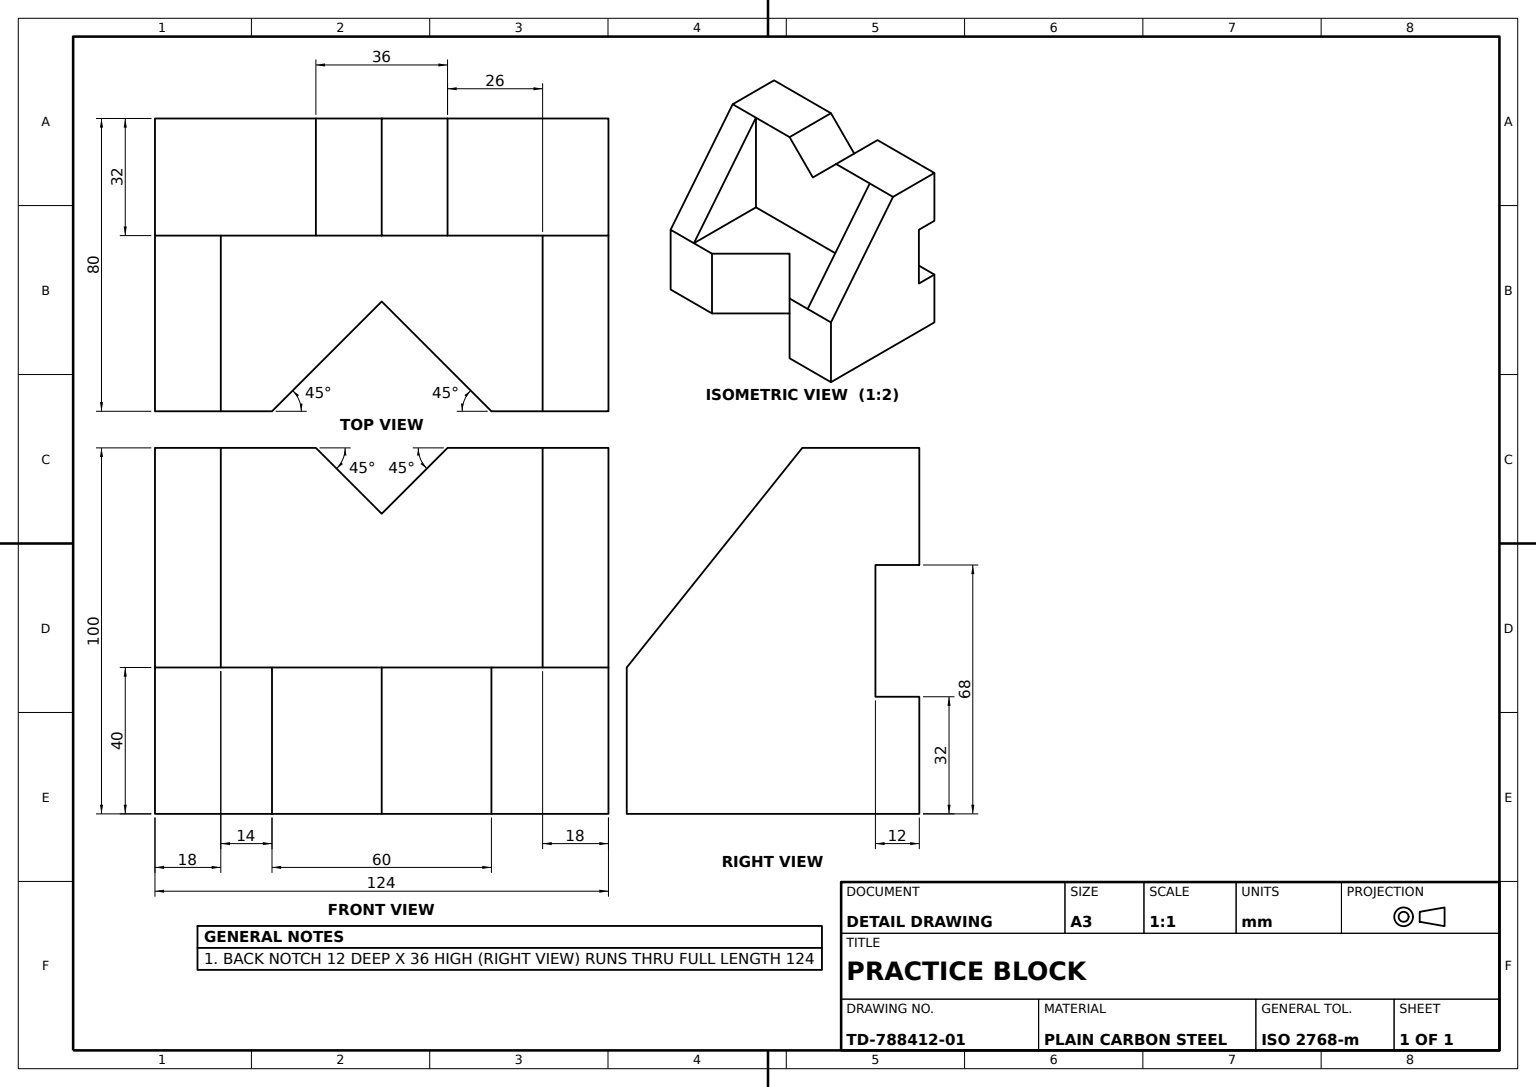
from build123d import *

# Parameters (mm, degrees)
BASE_PROFILE_SKETCH_W = 124
BASE_PROFILE_SKETCH_H = 100
BASE_BLOCK_32_DEPTH   = 32
FRONT_NOTCH_SKETCH_W  = 12
FRONT_NOTCH_SKETCH_H  = 36
FRONT_NOTCH_CUT_DEPTH = 124
UPRIGHT_WALL_SKETCH_W = 124
UPRIGHT_WALL_SKETCH_H = 48
UPRIGHT_WALL_40_DEPTH = 40
WEDGE_A_18_DEPTH      = 18
WEDGE_B_18_DEPTH      = 18
V_NOTCH_CUT_DEPTH     = 40
SIDE_SLOT_CUT_DEPTH   = 40


with BuildPart() as part:
    # Base Profile Sketch → Base Block 32 (new body)
    with BuildSketch(Plane.XY):
        with Locations((62, -50)):
            Rectangle(BASE_PROFILE_SKETCH_W, BASE_PROFILE_SKETCH_H)
    extrude(amount=BASE_BLOCK_32_DEPTH)

    # Front Notch Sketch → Front Notch Cut (cut)
    with BuildSketch(Plane.ZY):
        with Locations((6, -50)):
            Rectangle(FRONT_NOTCH_SKETCH_W, FRONT_NOTCH_SKETCH_H)
    extrude(amount=-FRONT_NOTCH_CUT_DEPTH, mode=Mode.SUBTRACT)

    # Upright Wall Sketch → Upright Wall 40 (add)
    with BuildSketch(Plane.XZ.offset(100)):
        with Locations((62, 56)):
            Rectangle(UPRIGHT_WALL_SKETCH_W, UPRIGHT_WALL_SKETCH_H)
    extrude(amount=-UPRIGHT_WALL_40_DEPTH)

    # Wedge A Sketch → Wedge A 18 (add)
    with BuildSketch(Plane(origin=(124, 0, 0), x_dir=(0, 0, -1), z_dir=(1, 0, 0))):
        Polygon((-80, -60), (-32, 0), (-32, -60), align=None)
    extrude(amount=-WEDGE_A_18_DEPTH)

    # Wedge B Sketch → Wedge B 18 (add)
    with BuildSketch(Plane.ZY):
        Polygon((80, -60), (32, 0), (32, -60), align=None)
    extrude(amount=-WEDGE_B_18_DEPTH)

    # V Notch Sketch → V Notch Cut (cut)
    with BuildSketch(Plane(origin=(0, -60, 0), x_dir=(1, 0, 0), z_dir=(0, 1, 0))):
        Polygon((32, -80), (62, -80), (92, -80), (62, -50), align=None)
    extrude(amount=-V_NOTCH_CUT_DEPTH, mode=Mode.SUBTRACT)

    # Side Slot Sketch → Side Slot Cut (cut)
    with BuildSketch(Plane.XY.offset(32)):
        Polygon((80, 0), (62, 0), (44, 0), (62, -18), align=None)
    extrude(amount=-SIDE_SLOT_CUT_DEPTH, mode=Mode.SUBTRACT)


solid = part.part
